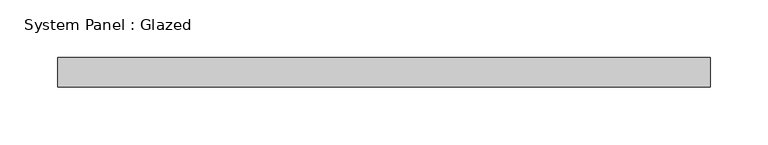
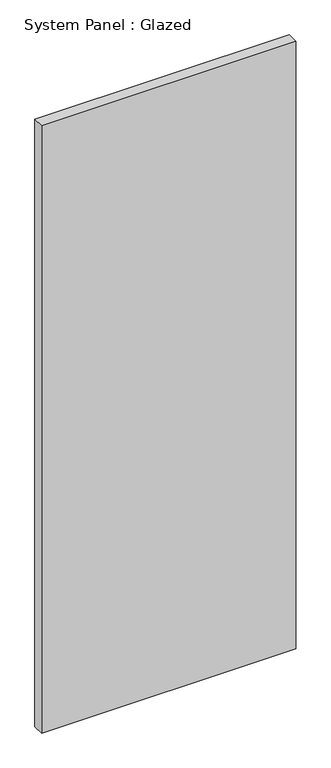
"""IFC4 building model written with IfcOpenShell, lengths in millimetres: plate geometry, System Panel : Glazed."""

from ifc_helpers import new_model, si_unit, origin, origin_with_axes, place, context, project, spatial, polyline, outline, extrude, source, transform, mapped, element, save


def system_panel_glazed_32442be8(model_context):
    return source(origin(), model_context, "Body", "SweptSolid", [
        extrude(outline(polyline([(282.575, 19.05), (-282.575, 19.05), (-282.575, 44.45), (282.575, 44.45), (282.575, 19.05)])), origin_with_axes(), (0.0, 0.0, 1.0), 1426.4572054),
    ])


if __name__ == "__main__":
    model = new_model("IFC4")
    model_context = context("Model", 3, world=origin())
    ifc_project = project(units=[si_unit("LENGTHUNIT", "METRE", prefix="MILLI")], contexts=[model_context])
    site = spatial("IfcSite", under=ifc_project)
    building = spatial("IfcBuilding", under=site)
    placement = place(None, origin())
    system_panel_glazed_shape = system_panel_glazed_32442be8(model_context)
    element("IfcPlate", 1, ObjectType="System Panel : Glazed", at=placement, inside=building, context=model_context, shape_type="MappedRepresentation", body=[
        mapped(system_panel_glazed_shape, transform((0.0, 0.0, 0.0), x_axis=(1.0, 0.0, 0.0), y_axis=(0.0, 1.0, 0.0), z_axis=(0.0, 0.0, 1.0))),
    ])
    save(model, "model.ifc")

# Revit data of these elements
# Type "System Panel : Glazed"
#   Construction Type Id = "GSP4R"
#   Analytic Construction = "1/8 in Pilkington single glazing"
#   Visual Light Transmittance = 0.9
#   Solar Heat Gain Coefficient = 0.86
#   Heat Transfer Coefficient (U) = 1.18115 BTU/(h·ft²·°F)
#   Define Thermal Properties by = 1
# Element 1 (IfcPlate, "System Panel : Glazed")
#   Materials on its faces: "Glass"
# Materials
#   "Glass": class "Glass", colour RGB 0 128 192, transparency 0.75, Description = "Soda Lime Glass", Cost = 0
